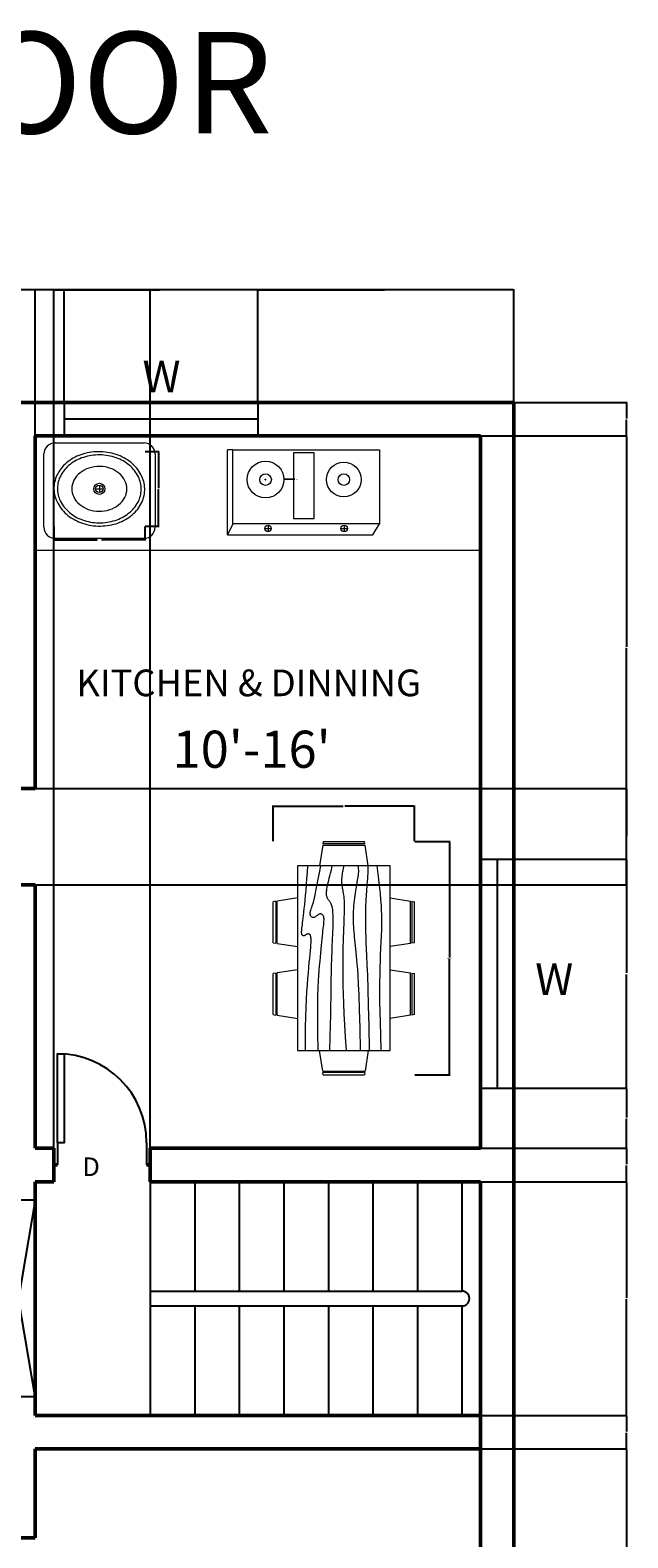
# Model space of a CAD drawing. Units: inches. Extents: x 2164 to 3752, y 2015 to 2629.
# Tile 4 of 8: x 2461 to 2622, y 2223 to 2629. Entities that reach past the tile are written whole.
import ezdxf
from ezdxf.enums import TextEntityAlignment as Align

# ---------------------------------------------------------------- set-up
doc = ezdxf.new("R2010")
doc.units = ezdxf.units.IN
for name, color, linetype, lineweight in [('A-ANNO-DIMS', 2, 'Continuous', 18), ('A-ANNO-TEXT', 7, 'Continuous', 25), ('A-AREA-IDEN', 3, 'Continuous', 25), ('A-DOOR', 3, 'Continuous', 25), ('A-FLOR-FIXT', 8, 'Continuous', 18), ('A-FLOR-STRS', 2, 'Continuous', 25), ('A-FURN', 8, 'Continuous', 18), ('A-GLAZ', 4, 'Continuous', 25), ('A-WALL', 7, 'Continuous', 50)]:
    doc.layers.add(name, color=color, linetype=linetype, lineweight=lineweight)
doc.styles.get("Standard").update_dxf_attribs({"font": 'arial.ttf'})
doc.dimstyles.get("Standard").update_dxf_attribs({"dimtxt": 0.18, "dimasz": 0.18, "dimexe": 0.18, "dimexo": 0.0625, "dimgap": 0.09, "dimtad": 0, "dimtih": 1, "dimtoh": 1, "dimdec": 4, "dimzin": 0, "dimdsep": 46, "dimtxsty": 'Standard', "dimcen": 0.09, "dimadec": 0, "dimazin": 0, "dimtfac": 1, "dimtdec": 4, "dimtofl": 0, "dimtmove": 0, "dimatfit": 3, "dimfxl": 1, "dimtolj": 1, "dimtzin": 0, "dimarcsym": 0})

# ---------------------------------------------------------------- blocks, each defined once
blk = doc.blocks.new('Dining Set - 36 x 72 in.')
for p, q in [((-22.2343, 26.00059), (-23.4847, 17.99762)), ((-22.2304, 26), (-5.7608, 26)), ((-22, 27.5), (-22.1562, 26.50042)), ((-5.8416, 26.5), (-22.1534, 26.5)), ((-22, 27.5), (-6, 27.5)), ((-5.8437, 26.49966), (-6, 27.5)), ((-4.5152, 17.99762), (-5.7655, 25.99926)), ((5.7657, 26.00059), (4.5153, 17.99762)), ((5.7696, 26), (22.2392, 26)), ((6, 27.5), (5.8438, 26.50042)), ((22.1584, 26.5), (5.8466, 26.5)), ((6, 27.5), (22, 27.5)), ((22.1563, 26.49966), (22, 27.5)), ((23.4848, 17.99762), (22.2345, 25.99926)), ((36, 18), (-36, 18)), ((-36, 18), (-36, -18)), ((36, -18), (36, 18)), ((-45.5, 8), (-44.5004, 8.15617)), ((-45.5, 8), (-45.5, -8)), ((-44.5, -8.15843), (-44.5, 8.15338)), ((-44.0006, 8.23428), (-35.9976, 9.48474)), ((-44, 8.23041), (-44, -8.23915)), ((44.0006, 8.23428), (35.9976, 9.48474)), ((44, 8.23041), (44, -8.23915)), ((44.5, -8.15843), (44.5, 8.15338)), ((45.5, 8), (44.5005, 8.15617)), ((45.5, 8), (45.5, -8)), ((-44.4997, -8.15631), (-45.5, -8)), ((-35.9976, -9.48476), (-43.9993, -8.2345)), ((35.9976, -9.48476), (43.9993, -8.2345)), ((44.4997, -8.15631), (45.5, -8)), ((-36, -18), (36, -18)), ((-22.2343, -26.0006), (-23.4847, -17.99762)), ((-4.5152, -17.99762), (-5.7655, -25.99928)), ((5.7657, -26.0006), (4.5153, -17.99762)), ((23.4848, -17.99762), (22.2345, -25.99928)), ((-22.2304, -26), (-5.7608, -26)), ((-22, -27.5), (-22.1562, -26.50044)), ((-5.8416, -26.5), (-22.1534, -26.5)), ((-22, -27.5), (-6, -27.5)), ((-5.8437, -26.49967), (-6, -27.5)), ((5.7696, -26), (22.2392, -26)), ((6, -27.5), (5.8438, -26.50044)), ((22.1584, -26.5), (5.8466, -26.5)), ((6, -27.5), (22, -27.5)), ((22.1563, -26.49967), (22, -27.5))]:
    blk.add_line(p, q)
for points in [[(-36, 15), (-31.1772, 14.97754), (-26.8079, 14.91406), (-22.8538, 14.81543), (-19.276, 14.6875), (-16.0362, 14.53613), (-13.0957, 14.36718), (-10.4159, 14.18652), (-7.9583, 14), (-5.6904, 13.81315), (-3.6035, 13.63021), (-1.6954, 13.45508), (0.0365, 13.29166), (1.5945, 13.14388), (2.9811, 13.01562), (4.1988, 12.9108), (5.25, 12.83333), (6.1393, 12.78613), (6.8802, 12.76823), (7.4883, 12.77767), (7.9792, 12.8125), (8.3685, 12.87077), (8.6719, 12.95052), (8.9049, 13.0498), (9.0833, 13.16666), (9.2205, 13.29899), (9.3216, 13.44401), (9.3895, 13.59879), (9.4271, 13.76041), (9.4373, 13.92594), (9.4232, 14.09245), (9.3875, 14.257), (9.3333, 14.41666), (9.2638, 14.56917), (9.1836, 14.71484), (9.0975, 14.85465), (9.0104, 14.98958), (8.9272, 15.1206), (8.8529, 15.2487), (8.7922, 15.37483), (8.75, 15.5), (8.7305, 15.62467), (8.7344, 15.74739), (8.7617, 15.86621), (8.8125, 15.97916), (8.8867, 16.08431), (8.9844, 16.17968), (9.1055, 16.26334), (9.25, 16.33333), (9.4189, 16.38802), (9.6172, 16.42708), (9.8506, 16.45052), (10.125, 16.45833), (10.4463, 16.45052), (10.8203, 16.42708), (11.2529, 16.38802), (11.75, 16.33333), (12.3184, 16.26318), (12.9694, 16.17838), (13.7151, 16.07991), (14.5677, 15.96875), (15.5395, 15.84586), (16.6426, 15.71224), (17.8893, 15.56884), (19.2917, 15.41666), (20.859, 15.25667), (22.5879, 15.08984), (24.4721, 14.91715), (26.5052, 14.73958), (28.6809, 14.5581), (30.9929, 14.3737), (33.4347, 14.18733), (36, 14)], [(-36, 10), (-28.9766, 10.14274), (-23.1725, 10.20442), (-18.4241, 10.19775), (-14.5677, 10.13541), (-11.4399, 10.03011), (-8.877, 9.89453), (-6.7154, 9.74137), (-4.7917, 9.58333), (-2.9698, 9.43082), (-1.2246, 9.28515), (0.4415, 9.14534), (2.026, 9.01041), (3.5266, 8.87939), (4.9408, 8.7513), (6.266, 8.62516), (7.5, 8.5), (8.6411, 8.37549), (9.6914, 8.2539), (10.6538, 8.13818), (11.5312, 8.03125), (12.3267, 7.93603), (13.043, 7.85547), (13.6831, 7.79248), (14.25, 7.75), (14.7471, 7.7303), (15.1797, 7.73307), (15.5537, 7.75732), (15.875, 7.80208), (16.1494, 7.86637), (16.3828, 7.94922), (16.5811, 8.04964), (16.75, 8.16666), (16.8944, 8.29915), (17.0143, 8.44531), (17.1089, 8.60319), (17.1771, 8.77083), (17.218, 8.94629), (17.2305, 9.1276), (17.2137, 9.31282), (17.1667, 9.5), (17.0895, 9.6875), (16.987, 9.875), (16.8649, 10.0625), (16.7292, 10.25), (16.5856, 10.4375), (16.4401, 10.625), (16.2985, 10.8125), (16.1667, 11), (16.05, 11.18733), (15.9518, 11.3737), (15.8752, 11.5581), (15.8229, 11.73958), (15.798, 11.91715), (15.8034, 12.08984), (15.842, 12.25667), (15.9167, 12.41666), (16.0295, 12.56836), (16.1784, 12.70833), (16.3605, 12.83268), (16.5729, 12.9375), (16.8127, 13.01888), (17.0768, 13.07291), (17.3625, 13.0957), (17.6667, 13.08333), (17.9894, 13.03312), (18.3418, 12.94726), (18.7382, 12.82918), (19.1927, 12.68229), (19.7195, 12.51001), (20.3327, 12.31575), (21.0465, 12.10294), (21.875, 11.875), (22.8357, 11.63354), (23.959, 11.37304), (25.2786, 11.08618), (26.8282, 10.76562), (28.6414, 10.40405), (30.752, 9.99414), (33.1936, 9.52856), (36, 9)], [(-36, 5.5), (-30.7157, 5.3348), (-26.069, 5.20963), (-21.9946, 5.11767), (-18.4271, 5.05208), (-15.3009, 5.00602), (-12.5508, 4.97265), (-10.1112, 4.94515), (-7.9167, 4.91666), (-5.909, 4.88167), (-4.0586, 4.83984), (-2.3429, 4.79215), (-0.7396, 4.73958), (0.7739, 4.6831), (2.22, 4.6237), (3.6213, 4.56233), (5, 4.5), (6.373, 4.43782), (7.7344, 4.3776), (9.0723, 4.32129), (10.375, 4.27083), (11.6309, 4.22819), (12.8281, 4.19531), (13.9551, 4.17415), (15, 4.16666), (15.954, 4.17448), (16.819, 4.19791), (17.6001, 4.23698), (18.3021, 4.29166), (18.9299, 4.36198), (19.4883, 4.44791), (19.9823, 4.54948), (20.4167, 4.66666), (20.7969, 4.79899), (21.1302, 4.94401), (21.4245, 5.09879), (21.6875, 5.26041), (21.9271, 5.42594), (22.1511, 5.59245), (22.3672, 5.757), (22.5834, 5.91666), (22.8065, 6.06868), (23.0404, 6.21093), (23.2879, 6.34147), (23.5521, 6.45833), (23.8358, 6.55957), (24.142, 6.64323), (24.4735, 6.70735), (24.8334, 6.75), (25.2235, 6.76969), (25.642, 6.76692), (26.0858, 6.74267), (26.5521, 6.69791), (27.0379, 6.63362), (27.5404, 6.55078), (28.0565, 6.45036), (28.5834, 6.33333), (29.1242, 6.19987), (29.7071, 6.04687), (30.3661, 5.87044), (31.1354, 5.66666), (32.0493, 5.43164), (33.142, 5.16146), (34.4475, 4.85221), (36, 4.5)], [(-36, -1), (-30.7915, -0.6591), (-26.0195, -0.38216), (-21.6519, -0.16284), (-17.6563, 0.00521), (-14.0005, 0.12833), (-10.6523, 0.21289), (-7.5796, 0.26522), (-4.75, 0.29166), (-2.134, 0.29793), (0.2878, 0.28711), (2.5317, 0.26163), (4.6146, 0.22396), (6.5529, 0.17651), (8.3633, 0.12174), (10.0623, 0.06209), (11.6667, 0), (13.1899, -0.06201), (14.6341, -0.1211), (15.9982, -0.17432), (17.2813, -0.21875), (18.4823, -0.25147), (19.6003, -0.26953), (20.6343, -0.27002), (21.5834, -0.25), (22.4481, -0.20768), (23.2357, -0.14584), (23.9549, -0.06836), (24.6146, 0.02083), (25.2235, 0.11784), (25.7904, 0.21875), (26.3241, 0.31966), (26.8334, 0.41666), (27.3265, 0.50618), (27.8099, 0.58593), (28.2894, 0.65397), (28.7709, 0.70833), (29.2601, 0.74707), (29.763, 0.76823), (30.2855, 0.76985), (30.8334, 0.75), (31.4088, 0.70784), (31.9994, 0.64713), (32.589, 0.57275), (33.1615, 0.48958), (33.7008, 0.4025), (34.1908, 0.3164), (34.6153, 0.23616), (34.9584, 0.16666), (35.2099, 0.11165), (35.3848, 0.07031), (35.504, 0.04069), (35.5886, 0.02083), (35.6594, 0.00879), (35.7377, 0.0026), (35.8442, 0.00032), (36, 0)], [(-36, -6.5), (-27.1843, -6.31267), (-20.084, -6.1263), (-14.469, -5.9419), (-10.1094, -5.76042), (-6.7752, -5.58285), (-4.2363, -5.41016), (-2.2629, -5.24333), (-0.625, -5.08334), (0.8708, -4.93099), (2.2715, -4.78646), (3.5872, -4.64974), (4.8281, -4.52084), (6.0046, -4.39974), (7.127, -4.28646), (8.2053, -4.18099), (9.25, -4.08334), (10.2705, -3.99382), (11.2734, -3.91407), (12.2647, -3.84603), (13.25, -3.79167), (14.2354, -3.75293), (15.2266, -3.73177), (16.2295, -3.73015), (17.25, -3.75), (18.2912, -3.79248), (19.3451, -3.85547), (20.4009, -3.93604), (21.4479, -4.03125), (22.4754, -4.13819), (23.4727, -4.25391), (24.4289, -4.37549), (25.3334, -4.5), (26.1785, -4.62492), (26.9694, -4.74935), (27.7145, -4.87281), (28.4219, -4.99479), (29.1, -5.11483), (29.7572, -5.23242), (30.4016, -5.34709), (31.0417, -5.45834), (31.6837, -5.56437), (32.3262, -5.65821), (32.9658, -5.73153), (33.599, -5.77604), (34.2224, -5.78345), (34.8327, -5.74545), (35.4264, -5.65373), (36, -5.5)], [(-36, -10), (-26.4022, -9.81299), (-18.4675, -9.62891), (-11.9839, -9.45069), (-6.7396, -9.28125), (-2.5226, -9.12354), (0.8789, -8.98047), (3.6769, -8.85498), (6.0833, -8.75), (8.2767, -8.66765), (10.3021, -8.60677), (12.1712, -8.56543), (13.8958, -8.54167), (15.4876, -8.53353), (16.9583, -8.53907), (18.3197, -8.55632), (19.5834, -8.58334), (20.7616, -8.61841), (21.8685, -8.66081), (22.9188, -8.71004), (23.9271, -8.76563), (24.9081, -8.82707), (25.8763, -8.89388), (26.8465, -8.96558), (27.8334, -9.04167), (28.8474, -9.12118), (29.8828, -9.20117), (30.93, -9.27824), (31.9792, -9.34896), (33.0205, -9.40991), (34.0443, -9.45768), (35.0407, -9.48885), (36, -9.5)], [(-36, -14.5), (-30.0881, -14.33513), (-25.0332, -14.21224), (-20.7312, -14.12647), (-17.0781, -14.07292), (-13.97, -14.04671), (-11.3027, -14.04297), (-8.9724, -14.05681), (-6.875, -14.08334), (-4.9224, -14.11833), (-3.0905, -14.16016), (-1.3709, -14.20785), (0.2448, -14.26042), (1.7647, -14.3169), (3.1973, -14.3763), (4.5507, -14.43767), (5.8333, -14.5), (7.0554, -14.5621), (8.235, -14.62175), (9.3922, -14.67652), (10.5469, -14.72396), (11.7192, -14.76164), (12.929, -14.78711), (14.1965, -14.79794), (15.5417, -14.79167), (16.9933, -14.76424), (18.6152, -14.70508), (20.4804, -14.60197), (22.6615, -14.44271), (25.2312, -14.21509), (28.2624, -13.9069), (31.8277, -13.50594), (36, -13)]]:
    blk.add_lwpolyline(points)
blk = doc.blocks.new('Sink - Oval top')
for p, q in [((-1, 0), (1, 0)), ((0, 1), (0, -1))]:
    blk.add_line(p, q)
for points in [[(-12.23, 0.39, 0.117634), (-11.46, -3.36, 0.104469), (-8.88, -6.8, 0.090016), (-5.08, -9.07, 0.08192), (-0.32, -10.02, 0.08192), (4.49, -9.38, 0.090016), (8.42, -7.36, 0.104469), (11.22, -4.09, 0.117634), (12.23, -0.39, 0.117634), (11.46, 3.36, 0.104469), (8.88, 6.8, 0.090016), (5.08, 9.07, 0.08192), (0.32, 10.02, 0.08192), (-4.49, 9.38, 0.090016), (-8.42, 7.36, 0.104469), (-11.22, 4.09, 0.117634)], [(-11.29, 0.16, 0.118622), (-10.52, -3.25, 0.104678), (-8.07, -6.36, 0.089562), (-4.54, -8.37, 0.081185), (-0.13, -9.15, 0.081185), (4.3, -8.49, 0.089562), (7.89, -6.58, 0.104678), (10.42, -3.55, 0.118622), (11.29, -0.16, 0.118622), (10.52, 3.25, 0.104678), (8.07, 6.36, 0.089562), (4.54, 8.37, 0.081185), (0.13, 9.15, 0.081185), (-4.3, 8.49, 0.089562), (-7.89, 6.58, 0.104678), (-10.42, 3.55, 0.118622)], [(-7.42, 0.08, 0.118283), (-6.91, -2.17, 0.104607), (-5.29, -4.21, 0.089718), (-2.97, -5.53, 0.081436), (-0.07, -6.04, 0.081436), (2.84, -5.59, 0.089718), (5.2, -4.33, 0.104607), (6.86, -2.32, 0.118283), (7.42, -0.08, 0.118283), (6.91, 2.17, 0.104607), (5.29, 4.21, 0.089718), (2.97, 5.53, 0.081436), (0.07, 6.04, 0.081436), (-2.84, 5.59, 0.089718), (-5.2, 4.33, 0.104607), (-6.86, 2.32, 0.118283)]]:
    blk.add_lwpolyline(points, format="xyb", close=True)
for radius in [1.5, 1]:
    blk.add_circle((0, 0), radius)
blk = doc.blocks.new('*U2')
for p, q in [((0, 0), (0, -6)), ((24, 0), (24, -6))]:
    blk.add_line(p, q)
blk.add_lwpolyline([(0, 0), (0, 24), (1.75, 24), (1.75, 0)], close=True)
blk.add_arc((0, 0), 24, 0, 90)
blk = doc.blocks.new('STAIR-HANDRAIL')
for p, q in [((84, 63), (84, 33.5)), ((0, 33.5), (84, 33.5)), ((0, 29.5), (84, 29.5)), ((84, 29.5), (84, 0))]:
    blk.add_line(p, q)
blk.add_arc((84, 31.5), 2, 270, 90)
blk = doc.blocks.new('VENT-OPENING')
for p, q in [((9, 53), (0, 53)), ((9, 53), (0, 0)), ((9, 0), (0, 53)), ((9, 0), (0, 0))]:
    blk.add_line(p, q)
blk = doc.blocks.new('*D37')
at = {"layer": 'A-ANNO-DIMS', "color": 0, "lineweight": -2, "transparency": 16777216}
for p, q in [((2564.38, 2410.45), (2573.95, 2410.45)), ((2573.77, 2410.27), (2573.77, 2379.15)), ((2573.77, 2347.66), (2573.77, 2378.78)), ((2564.38, 2347.48), (2573.95, 2347.48))]:
    blk.add_line(p, q, dxfattribs=at)
at = {"layer": 'A-ANNO-DIMS', "color": 0, "transparency": 16777216}
for points in [[(2573.74, 2410.27), (2573.8, 2410.27), (2573.77, 2410.45)], [(2573.74, 2347.66), (2573.8, 2347.66), (2573.77, 2347.48)]]:
    blk.add_solid(points, dxfattribs=at)
at = {"layer": 'Defpoints', "color": 0, "transparency": 16777216}
for p in [(2564.32, 2410.45), (2573.77, 2410.45), (2564.32, 2347.48)]:
    blk.add_point(p, dxfattribs=at)
at = {"layer": 'A-ANNO-DIMS', "color": 0, "transparency": 16777216, "insert": (2573.77, 2378.96), "char_height": 0.18, "attachment_point": 5}
blk.add_mtext('\\A1;DINING SET 63', dxfattribs=at)
blk = doc.blocks.new('*D38')
at = {"layer": 'A-ANNO-DIMS', "color": 0, "lineweight": -2, "transparency": 16777216}
for p, q in [((2526.26, 2410.51), (2526.26, 2420.07)), ((2526.44, 2419.89), (2545.07, 2419.89)), ((2564.14, 2419.89), (2545.51, 2419.89)), ((2564.32, 2410.51), (2564.32, 2420.07))]:
    blk.add_line(p, q, dxfattribs=at)
at = {"layer": 'A-ANNO-DIMS', "color": 0, "transparency": 16777216}
for points in [[(2526.44, 2419.92), (2526.44, 2419.86), (2526.26, 2419.89)], [(2564.14, 2419.92), (2564.14, 2419.86), (2564.32, 2419.89)]]:
    blk.add_solid(points, dxfattribs=at)
at = {"layer": 'Defpoints', "color": 0, "transparency": 16777216}
for p in [(2526.26, 2419.89), (2526.26, 2410.45), (2564.32, 2410.45)]:
    blk.add_point(p, dxfattribs=at)
at = {"layer": 'A-ANNO-DIMS', "color": 0, "transparency": 16777216, "insert": (2545.29, 2419.89), "char_height": 0.18, "attachment_point": 5}
blk.add_mtext('\\A1;38', dxfattribs=at)
blk = doc.blocks.new('*D39')
at = {"layer": 'A-ANNO-DIMS', "color": 0, "lineweight": -2, "transparency": 16777216}
for p, q in [((2467.11, 2495.33), (2467.11, 2491.52)), ((2491.66, 2495.33), (2491.66, 2491.52)), ((2467.29, 2491.7), (2478.83, 2491.7)), ((2491.48, 2491.7), (2479.93, 2491.7))]:
    blk.add_line(p, q, dxfattribs=at)
at = {"layer": 'A-ANNO-DIMS', "color": 0, "transparency": 16777216}
for points in [[(2467.29, 2491.73), (2467.29, 2491.67), (2467.11, 2491.7)], [(2491.48, 2491.73), (2491.48, 2491.67), (2491.66, 2491.7)]]:
    blk.add_solid(points, dxfattribs=at)
at = {"layer": 'Defpoints', "color": 0, "transparency": 16777216}
for p in [(2467.11, 2495.39), (2491.66, 2495.39), (2491.66, 2491.7)]:
    blk.add_point(p, dxfattribs=at)
at = {"layer": 'A-ANNO-DIMS', "color": 0, "transparency": 16777216, "insert": (2479.38, 2491.7), "char_height": 0.18, "attachment_point": 5}
blk.add_mtext('\\A1;SINK 25', dxfattribs=at)
blk = doc.blocks.new('*D40')
at = {"layer": 'A-ANNO-DIMS', "color": 0, "lineweight": -2, "transparency": 16777216}
for p, q in [((2491.72, 2515.52), (2495.52, 2515.52)), ((2495.34, 2515.34), (2495.34, 2505.64)), ((2495.34, 2495.57), (2495.34, 2505.27)), ((2491.72, 2495.39), (2495.52, 2495.39))]:
    blk.add_line(p, q, dxfattribs=at)
at = {"layer": 'A-ANNO-DIMS', "color": 0, "transparency": 16777216}
for points in [[(2495.31, 2515.34), (2495.37, 2515.34), (2495.34, 2515.52)], [(2495.31, 2495.57), (2495.37, 2495.57), (2495.34, 2495.39)]]:
    blk.add_solid(points, dxfattribs=at)
at = {"layer": 'Defpoints', "color": 0, "transparency": 16777216}
for p in [(2491.66, 2515.52), (2495.34, 2515.52), (2491.66, 2495.39)]:
    blk.add_point(p, dxfattribs=at)
at = {"layer": 'A-ANNO-DIMS', "color": 0, "transparency": 16777216, "insert": (2495.34, 2505.46), "char_height": 0.18, "attachment_point": 5}
blk.add_mtext('\\A1;20', dxfattribs=at)
blk = doc.blocks.new('*D51')
at = {"layer": 'A-ANNO-DIMS', "color": 0, "lineweight": -2, "transparency": 16777216}
for p, q in [((2438.92, 2528.78), (2438.92, 2559.25)), ((2439.1, 2559.07), (2453.99, 2559.07)), ((2469.68, 2559.07), (2454.78, 2559.07)), ((2469.86, 2528.78), (2469.86, 2559.25))]:
    blk.add_line(p, q, dxfattribs=at)
at = {"layer": 'A-ANNO-DIMS', "color": 0, "transparency": 16777216}
for points in [[(2439.1, 2559.1), (2439.1, 2559.04), (2438.92, 2559.07)], [(2469.68, 2559.1), (2469.68, 2559.04), (2469.86, 2559.07)]]:
    blk.add_solid(points, dxfattribs=at)
at = {"layer": 'Defpoints', "color": 0, "transparency": 16777216}
for p in [(2469.86, 2559.07), (2438.92, 2528.72), (2469.86, 2528.72)]:
    blk.add_point(p, dxfattribs=at)
at = {"layer": 'A-ANNO-DIMS', "color": 0, "transparency": 16777216, "insert": (2454.39, 2559.07), "char_height": 0.18, "attachment_point": 5}
blk.add_mtext('\\A1;30.94', dxfattribs=at)
blk = doc.blocks.new('*D52')
at = {"layer": 'A-ANNO-DIMS', "color": 0, "lineweight": -2, "transparency": 16777216}
for p, q in [((2469.86, 2528.78), (2469.86, 2559.25)), ((2470.04, 2559.07), (2495.59, 2559.07)), ((2521.89, 2559.07), (2496.34, 2559.07)), ((2522.07, 2528.78), (2522.07, 2559.25))]:
    blk.add_line(p, q, dxfattribs=at)
at = {"layer": 'A-ANNO-DIMS', "color": 0, "transparency": 16777216}
for points in [[(2470.04, 2559.1), (2470.04, 2559.04), (2469.86, 2559.07)], [(2521.89, 2559.1), (2521.89, 2559.04), (2522.07, 2559.07)]]:
    blk.add_solid(points, dxfattribs=at)
at = {"layer": 'Defpoints', "color": 0, "transparency": 16777216}
for p in [(2522.07, 2559.07), (2469.86, 2528.72), (2522.07, 2528.72)]:
    blk.add_point(p, dxfattribs=at)
at = {"layer": 'A-ANNO-DIMS', "color": 0, "transparency": 16777216, "insert": (2495.96, 2559.07), "char_height": 0.18, "attachment_point": 5}
blk.add_mtext('\\A1;52.21', dxfattribs=at)
blk = doc.blocks.new('*D53')
at = {"layer": 'A-ANNO-DIMS', "color": 0, "lineweight": -2, "transparency": 16777216}
for p, q in [((2522.07, 2528.78), (2522.07, 2559.25)), ((2522.25, 2559.07), (2556.2, 2559.07)), ((2590.93, 2559.07), (2556.98, 2559.07)), ((2591.11, 2528.78), (2591.11, 2559.25))]:
    blk.add_line(p, q, dxfattribs=at)
at = {"layer": 'A-ANNO-DIMS', "color": 0, "transparency": 16777216}
for points in [[(2522.25, 2559.1), (2522.25, 2559.04), (2522.07, 2559.07)], [(2590.93, 2559.1), (2590.93, 2559.04), (2591.11, 2559.07)]]:
    blk.add_solid(points, dxfattribs=at)
at = {"layer": 'Defpoints', "color": 0, "transparency": 16777216}
for p in [(2591.11, 2559.07), (2522.07, 2528.72), (2591.11, 2528.72)]:
    blk.add_point(p, dxfattribs=at)
at = {"layer": 'A-ANNO-DIMS', "color": 0, "transparency": 16777216, "insert": (2556.59, 2559.07), "char_height": 0.18, "attachment_point": 5}
blk.add_mtext('\\A1;69.04', dxfattribs=at)
blk = doc.blocks.new('*D54')
at = {"layer": 'A-ANNO-DIMS', "color": 0, "lineweight": -2, "transparency": 16777216}
for p, q in [((2195.11, 2528.78), (2195.11, 2559.25)), ((2195.29, 2559.07), (2392.82, 2559.07)), ((2590.93, 2559.07), (2393.4, 2559.07)), ((2591.11, 2528.78), (2591.11, 2559.25))]:
    blk.add_line(p, q, dxfattribs=at)
at = {"layer": 'A-ANNO-DIMS', "color": 0, "transparency": 16777216}
for points in [[(2195.29, 2559.1), (2195.29, 2559.04), (2195.11, 2559.07)], [(2590.93, 2559.1), (2590.93, 2559.04), (2591.11, 2559.07)]]:
    blk.add_solid(points, dxfattribs=at)
at = {"layer": 'Defpoints', "color": 0, "transparency": 16777216}
for p in [(2591.11, 2559.07), (2195.11, 2528.72), (2591.11, 2528.72)]:
    blk.add_point(p, dxfattribs=at)
at = {"layer": 'A-ANNO-DIMS', "color": 0, "transparency": 16777216, "insert": (2393.11, 2559.07), "char_height": 0.18, "attachment_point": 5}
blk.add_mtext('\\A1;396', dxfattribs=at)
blk = doc.blocks.new('*D58')
at = {"layer": 'A-ANNO-DIMS', "color": 0, "lineweight": -2, "transparency": 16777216}
for p, q in [((2453.11, 2519.78), (2453.11, 2559.25)), ((2453.29, 2559.07), (2457.46, 2559.07)), ((2461.93, 2559.07), (2457.76, 2559.07)), ((2462.11, 2519.78), (2462.11, 2559.25))]:
    blk.add_line(p, q, dxfattribs=at)
at = {"layer": 'A-ANNO-DIMS', "color": 0, "transparency": 16777216}
for points in [[(2453.29, 2559.1), (2453.29, 2559.04), (2453.11, 2559.07)], [(2461.93, 2559.1), (2461.93, 2559.04), (2462.11, 2559.07)]]:
    blk.add_solid(points, dxfattribs=at)
at = {"layer": 'Defpoints', "color": 0, "transparency": 16777216}
for p in [(2462.11, 2559.07), (2453.11, 2519.72), (2462.11, 2519.72)]:
    blk.add_point(p, dxfattribs=at)
at = {"layer": 'A-ANNO-DIMS', "color": 0, "transparency": 16777216, "insert": (2457.61, 2559.07), "char_height": 0.18, "attachment_point": 5}
blk.add_mtext('\\A1;9', dxfattribs=at)
blk = doc.blocks.new('*D79')
at = {"layer": 'A-ANNO-DIMS', "color": 0, "lineweight": -2, "transparency": 16777216}
for p, q in [((2582.17, 2246.72), (2621.64, 2246.72)), ((2621.46, 2246.54), (2621.46, 2206.1)), ((2621.46, 2165.31), (2621.46, 2205.74)), ((2591.17, 2165.13), (2621.64, 2165.13))]:
    blk.add_line(p, q, dxfattribs=at)
at = {"layer": 'A-ANNO-DIMS', "color": 0, "transparency": 16777216}
for points in [[(2621.43, 2246.54), (2621.49, 2246.54), (2621.46, 2246.72)], [(2621.43, 2165.31), (2621.49, 2165.31), (2621.46, 2165.13)]]:
    blk.add_solid(points, dxfattribs=at)
at = {"layer": 'Defpoints', "color": 0, "transparency": 16777216}
for p in [(2582.11, 2246.72), (2621.46, 2246.72), (2591.11, 2165.13)]:
    blk.add_point(p, dxfattribs=at)
at = {"layer": 'A-ANNO-DIMS', "color": 0, "transparency": 16777216, "insert": (2621.46, 2205.92), "char_height": 0.18, "attachment_point": 5}
blk.add_mtext('\\A1;81.59', dxfattribs=at)
blk = doc.blocks.new('*D80')
at = {"layer": 'A-ANNO-DIMS', "color": 0, "lineweight": -2, "transparency": 16777216}
for p, q in [((2582.17, 2255.72), (2621.64, 2255.72)), ((2621.46, 2255.54), (2621.46, 2251.4)), ((2621.46, 2246.9), (2621.46, 2251.04)), ((2582.17, 2246.72), (2621.64, 2246.72))]:
    blk.add_line(p, q, dxfattribs=at)
at = {"layer": 'A-ANNO-DIMS', "color": 0, "transparency": 16777216}
for points in [[(2621.43, 2255.54), (2621.49, 2255.54), (2621.46, 2255.72)], [(2621.43, 2246.9), (2621.49, 2246.9), (2621.46, 2246.72)]]:
    blk.add_solid(points, dxfattribs=at)
at = {"layer": 'Defpoints', "color": 0, "transparency": 16777216}
for p in [(2582.11, 2255.72), (2621.46, 2255.72), (2582.11, 2246.72)]:
    blk.add_point(p, dxfattribs=at)
at = {"layer": 'A-ANNO-DIMS', "color": 0, "transparency": 16777216, "insert": (2621.46, 2251.22), "char_height": 0.18, "attachment_point": 5}
blk.add_mtext('\\A1;9', dxfattribs=at)
blk = doc.blocks.new('*D81')
at = {"layer": 'A-ANNO-DIMS', "color": 0, "lineweight": -2, "transparency": 16777216}
for p, q in [((2582.17, 2318.72), (2621.64, 2318.72)), ((2621.46, 2318.54), (2621.46, 2287.4)), ((2621.46, 2255.9), (2621.46, 2287.04)), ((2582.17, 2255.72), (2621.64, 2255.72))]:
    blk.add_line(p, q, dxfattribs=at)
at = {"layer": 'A-ANNO-DIMS', "color": 0, "transparency": 16777216}
for points in [[(2621.43, 2318.54), (2621.49, 2318.54), (2621.46, 2318.72)], [(2621.43, 2255.9), (2621.49, 2255.9), (2621.46, 2255.72)]]:
    blk.add_solid(points, dxfattribs=at)
at = {"layer": 'Defpoints', "color": 0, "transparency": 16777216}
for p in [(2582.11, 2318.72), (2621.46, 2318.72), (2582.11, 2255.72)]:
    blk.add_point(p, dxfattribs=at)
at = {"layer": 'A-ANNO-DIMS', "color": 0, "transparency": 16777216, "insert": (2621.46, 2287.22), "char_height": 0.18, "attachment_point": 5}
blk.add_mtext('\\A1;63', dxfattribs=at)
blk = doc.blocks.new('*D82')
at = {"layer": 'A-ANNO-DIMS', "color": 0, "lineweight": -2, "transparency": 16777216}
for p, q in [((2582.17, 2327.72), (2621.64, 2327.72)), ((2621.46, 2327.54), (2621.46, 2323.4)), ((2621.46, 2318.9), (2621.46, 2323.04)), ((2582.17, 2318.72), (2621.64, 2318.72))]:
    blk.add_line(p, q, dxfattribs=at)
at = {"layer": 'A-ANNO-DIMS', "color": 0, "transparency": 16777216}
for points in [[(2621.43, 2327.54), (2621.49, 2327.54), (2621.46, 2327.72)], [(2621.43, 2318.9), (2621.49, 2318.9), (2621.46, 2318.72)]]:
    blk.add_solid(points, dxfattribs=at)
at = {"layer": 'Defpoints', "color": 0, "transparency": 16777216}
for p in [(2582.11, 2327.72), (2621.46, 2327.72), (2582.11, 2318.72)]:
    blk.add_point(p, dxfattribs=at)
at = {"layer": 'A-ANNO-DIMS', "color": 0, "transparency": 16777216, "insert": (2621.46, 2323.22), "char_height": 0.18, "attachment_point": 5}
blk.add_mtext('\\A1;9', dxfattribs=at)
blk = doc.blocks.new('*D83')
at = {"layer": 'A-ANNO-DIMS', "color": 0, "lineweight": -2, "transparency": 16777216}
for p, q in [((2591.17, 2343.89), (2621.64, 2343.89)), ((2621.46, 2343.71), (2621.46, 2335.98)), ((2621.46, 2327.9), (2621.46, 2335.62)), ((2582.17, 2327.72), (2621.64, 2327.72))]:
    blk.add_line(p, q, dxfattribs=at)
at = {"layer": 'A-ANNO-DIMS', "color": 0, "transparency": 16777216}
for points in [[(2621.43, 2343.71), (2621.49, 2343.71), (2621.46, 2343.89)], [(2621.43, 2327.9), (2621.49, 2327.9), (2621.46, 2327.72)]]:
    blk.add_solid(points, dxfattribs=at)
at = {"layer": 'Defpoints', "color": 0, "transparency": 16777216}
for p in [(2591.11, 2343.89), (2621.46, 2343.89), (2582.11, 2327.72)]:
    blk.add_point(p, dxfattribs=at)
at = {"layer": 'A-ANNO-DIMS', "color": 0, "transparency": 16777216, "insert": (2621.46, 2335.8), "char_height": 0.18, "attachment_point": 5}
blk.add_mtext('\\A1;16.17', dxfattribs=at)
blk = doc.blocks.new('*D84')
at = {"layer": 'A-ANNO-DIMS', "color": 0, "lineweight": -2, "transparency": 16777216}
for p, q in [((2591.17, 2405.68), (2621.64, 2405.68)), ((2621.46, 2405.5), (2621.46, 2374.97)), ((2621.46, 2344.07), (2621.46, 2374.6)), ((2591.17, 2343.89), (2621.64, 2343.89))]:
    blk.add_line(p, q, dxfattribs=at)
at = {"layer": 'A-ANNO-DIMS', "color": 0, "transparency": 16777216}
for points in [[(2621.43, 2405.5), (2621.49, 2405.5), (2621.46, 2405.68)], [(2621.43, 2344.07), (2621.49, 2344.07), (2621.46, 2343.89)]]:
    blk.add_solid(points, dxfattribs=at)
at = {"layer": 'Defpoints', "color": 0, "transparency": 16777216}
for p in [(2591.11, 2405.68), (2621.46, 2405.68), (2591.11, 2343.89)]:
    blk.add_point(p, dxfattribs=at)
at = {"layer": 'A-ANNO-DIMS', "color": 0, "transparency": 16777216, "insert": (2621.46, 2374.78), "char_height": 0.18, "attachment_point": 5}
blk.add_mtext('\\A1;61.8', dxfattribs=at)
blk = doc.blocks.new('*D85')
at = {"layer": 'A-ANNO-DIMS', "color": 0, "lineweight": -2, "transparency": 16777216}
for p, q in [((2582.17, 2519.72), (2621.64, 2519.72)), ((2621.46, 2519.54), (2621.46, 2462.88)), ((2621.46, 2405.86), (2621.46, 2462.52)), ((2591.17, 2405.68), (2621.64, 2405.68))]:
    blk.add_line(p, q, dxfattribs=at)
at = {"layer": 'A-ANNO-DIMS', "color": 0, "transparency": 16777216}
for points in [[(2621.43, 2519.54), (2621.49, 2519.54), (2621.46, 2519.72)], [(2621.43, 2405.86), (2621.49, 2405.86), (2621.46, 2405.68)]]:
    blk.add_solid(points, dxfattribs=at)
at = {"layer": 'Defpoints', "color": 0, "transparency": 16777216}
for p in [(2582.11, 2519.72), (2621.46, 2519.72), (2591.11, 2405.68)]:
    blk.add_point(p, dxfattribs=at)
at = {"layer": 'A-ANNO-DIMS', "color": 0, "transparency": 16777216, "insert": (2621.46, 2462.7), "char_height": 0.18, "attachment_point": 5}
blk.add_mtext('\\A1;114.04', dxfattribs=at)
blk = doc.blocks.new('*D86')
at = {"layer": 'A-ANNO-DIMS', "color": 0, "lineweight": -2, "transparency": 16777216}
for p, q in [((2591.17, 2528.72), (2621.64, 2528.72)), ((2621.46, 2528.54), (2621.46, 2524.4)), ((2621.46, 2519.9), (2621.46, 2524.04)), ((2582.17, 2519.72), (2621.64, 2519.72))]:
    blk.add_line(p, q, dxfattribs=at)
at = {"layer": 'A-ANNO-DIMS', "color": 0, "transparency": 16777216}
for points in [[(2621.43, 2528.54), (2621.49, 2528.54), (2621.46, 2528.72)], [(2621.43, 2519.9), (2621.49, 2519.9), (2621.46, 2519.72)]]:
    blk.add_solid(points, dxfattribs=at)
at = {"layer": 'Defpoints', "color": 0, "transparency": 16777216}
for p in [(2591.11, 2528.72), (2621.46, 2528.72), (2582.11, 2519.72)]:
    blk.add_point(p, dxfattribs=at)
at = {"layer": 'A-ANNO-DIMS', "color": 0, "transparency": 16777216, "insert": (2621.46, 2524.22), "char_height": 0.18, "attachment_point": 5}
blk.add_mtext('\\A1;9', dxfattribs=at)
blk = doc.blocks.new('*D95')
at = {"layer": 'A-ANNO-DIMS', "color": 0, "lineweight": -2, "transparency": 16777216}
for p, q in [((2467.11, 2327.78), (2467.11, 2559.25)), ((2467.29, 2559.07), (2479.89, 2559.07)), ((2492.93, 2559.07), (2480.33, 2559.07)), ((2493.11, 2327.78), (2493.11, 2559.25))]:
    blk.add_line(p, q, dxfattribs=at)
at = {"layer": 'A-ANNO-DIMS', "color": 0, "transparency": 16777216}
for points in [[(2467.29, 2559.1), (2467.29, 2559.04), (2467.11, 2559.07)], [(2492.93, 2559.1), (2492.93, 2559.04), (2493.11, 2559.07)]]:
    blk.add_solid(points, dxfattribs=at)
at = {"layer": 'Defpoints', "color": 0, "transparency": 16777216}
for p in [(2493.11, 2559.07), (2467.11, 2327.72), (2493.11, 2327.72)]:
    blk.add_point(p, dxfattribs=at)
at = {"layer": 'A-ANNO-DIMS', "color": 0, "transparency": 16777216, "insert": (2480.11, 2559.07), "char_height": 0.18, "attachment_point": 5}
blk.add_mtext('\\A1;26', dxfattribs=at)
blk = doc.blocks.new('*D97')
at = {"layer": 'A-ANNO-DIMS', "color": 0, "lineweight": -2, "transparency": 16777216}
for p, q in [((2462.17, 2424.72), (2621.64, 2424.72)), ((2621.46, 2424.54), (2621.46, 2411.9)), ((2621.46, 2398.9), (2621.46, 2411.54)), ((2462.17, 2398.72), (2621.64, 2398.72))]:
    blk.add_line(p, q, dxfattribs=at)
at = {"layer": 'A-ANNO-DIMS', "color": 0, "transparency": 16777216}
for points in [[(2621.43, 2424.54), (2621.49, 2424.54), (2621.46, 2424.72)], [(2621.43, 2398.9), (2621.49, 2398.9), (2621.46, 2398.72)]]:
    blk.add_solid(points, dxfattribs=at)
at = {"layer": 'Defpoints', "color": 0, "transparency": 16777216}
for p in [(2462.11, 2424.72), (2621.46, 2424.72), (2462.11, 2398.72)]:
    blk.add_point(p, dxfattribs=at)
at = {"layer": 'A-ANNO-DIMS', "color": 0, "transparency": 16777216, "insert": (2621.46, 2411.72), "char_height": 0.18, "attachment_point": 5}
blk.add_mtext('\\A1;26', dxfattribs=at)
blk = doc.blocks.new('*D150')
at = {"layer": 'A-ANNO-DIMS', "color": 0, "lineweight": -2, "transparency": 16777216}
for p, q in [((2524.1, 2507.96), (2524.28, 2507.96)), ((2524.19, 2507.87), (2524.19, 2508.05)), ((2532.11, 2508.03), (2529.32, 2508))]:
    blk.add_line(p, q, dxfattribs=at)
at = {"layer": 'A-ANNO-DIMS', "color": 0, "transparency": 16777216}
blk.add_solid([(2529.32, 2508.03), (2529.32, 2507.97), (2529.14, 2508)], dxfattribs=at)
at = {"layer": 'Defpoints', "color": 0, "transparency": 16777216}
for p in [(2519.23, 2507.91), (2529.14, 2508)]:
    blk.add_point(p, dxfattribs=at)
at = {"layer": 'A-ANNO-DIMS', "color": 0, "transparency": 16777216, "insert": (2532.6, 2508.03), "char_height": 0.18, "attachment_point": 5}
blk.add_mtext('\\A1;∅9.905', dxfattribs=at)

msp = doc.modelspace()

# ---------------------------------------------------------------- linework, layer by layer
at = {"layer": 'A-FLOR-FIXT'}
for p, q in [((2467.4392, 2517.854), (2491.4362, 2517.854)), ((2513.9601, 2493.0794), (2513.9601, 2515.9959)), ((2515.3902, 2515.9959), (2513.9601, 2515.9959)), ((2464.4392, 2495.0883), (2464.4392, 2514.854)), ((2494.4362, 2514.854), (2494.4362, 2495.0883)), ((2531.7072, 2515.1941), (2531.7072, 2497.5087)), ((2537.3015, 2515.1941), (2531.7072, 2515.1941)), ((2537.3015, 2497.5087), (2537.3015, 2515.1941)), ((2515.3902, 2496.0147), (2513.9601, 2493.0794)), ((2524.8551, 2495.6484), (2524.8551, 2493.926)), ((2531.7072, 2497.5087), (2537.3015, 2497.5087)), ((2545.3751, 2495.6484), (2545.3751, 2493.926)), ((2553.1059, 2493.0239), (2554.9364, 2496.0147)), ((2491.4362, 2492.0883), (2467.4392, 2492.0883)), ((2513.9601, 2493.0794), (2553.1059, 2493.0239)), ((2523.9939, 2494.7872), (2525.7163, 2494.7872)), ((2544.5139, 2494.7872), (2546.2363, 2494.7872)), ((2462.1113, 2488.9413), (2582.1113, 2488.9413))]:
    msp.add_line(p, q, dxfattribs=at)
msp.add_lwpolyline([(2515.3902, 2515.9959), (2554.9364, 2515.9959), (2554.9364, 2496.0147), (2515.3902, 2496.0147)], close=True, dxfattribs=at)
for centre, radius in [((2524.187, 2507.955), 4.9523), ((2545.2802, 2507.955), 4.6772), ((2524.187, 2507.955), 1.5591), ((2545.2802, 2507.955), 1.5591), ((2524.8551, 2494.7872), 0.8612), ((2545.3751, 2494.7872), 0.8612)]:
    msp.add_circle(centre, radius, dxfattribs=at)
for centre, start, end in [((2467.4392, 2514.854), 90, 180), ((2491.4362, 2514.854), 0, 90), ((2467.4392, 2495.0883), 180, 270), ((2491.4362, 2495.0883), 270, 0)]:
    msp.add_arc(centre, 3, start, end, dxfattribs=at)
at = {"layer": 'A-FLOR-STRS'}
for p, q in [((2493.1113, 2318.7172), (2493.1113, 2255.7172)), ((2505.1113, 2318.7172), (2505.1113, 2289.2172)), ((2517.1113, 2318.7172), (2517.1113, 2289.2172)), ((2529.1113, 2318.7172), (2529.1113, 2289.2172)), ((2541.1113, 2318.7172), (2541.1113, 2289.2172)), ((2553.1113, 2318.7172), (2553.1113, 2289.2172)), ((2565.1113, 2318.7172), (2565.1113, 2289.2172)), ((2505.1113, 2285.2172), (2505.1113, 2255.7172)), ((2517.1113, 2285.2172), (2517.1113, 2255.7172)), ((2529.1113, 2285.2172), (2529.1113, 2255.7172)), ((2541.1113, 2285.2172), (2541.1113, 2255.7172)), ((2553.1113, 2285.2172), (2553.1113, 2255.7172)), ((2565.1113, 2285.2172), (2565.1113, 2255.7172))]:
    msp.add_line(p, q, dxfattribs=at)
at = {"layer": 'A-GLAZ'}
for p, q in [((2469.8556, 2528.7172), (2469.8556, 2519.7172)), ((2522.0693, 2528.7172), (2522.1113, 2519.7172)), ((2522.0903, 2524.2172), (2469.8556, 2524.2172)), ((2582.1113, 2405.6818), (2591.1113, 2405.6818)), ((2586.6113, 2405.6818), (2586.6113, 2343.8868)), ((2582.1113, 2343.8868), (2591.1113, 2343.8868))]:
    msp.add_line(p, q, dxfattribs=at)
at = {"layer": 'A-WALL'}
for p, q in [((2195.1113, 2528.7172), (2591.1113, 2528.7172)), ((2591.1113, 2528.7172), (2591.1113, 2045.7172)), ((2462.1113, 2519.7172), (2582.1113, 2519.7172)), ((2462.1113, 2519.7172), (2462.1113, 2424.7172)), ((2582.1113, 2519.7172), (2582.1113, 2327.7172)), ((2453.1113, 2424.7172), (2462.1113, 2424.7172)), ((2453.1113, 2398.7172), (2462.1113, 2398.7172)), ((2462.1113, 2398.7172), (2462.1113, 2327.7172)), ((2462.1113, 2332.7172), (2462.1113, 2327.7172)), ((2462.1113, 2327.7172), (2467.1113, 2327.7172)), ((2467.1113, 2327.7172), (2467.1113, 2318.7172)), ((2493.1113, 2323.2172), (2493.1113, 2327.7172)), ((2493.1113, 2327.7172), (2582.1113, 2327.7172)), ((2467.1113, 2323.2172), (2468.1113, 2323.2172)), ((2492.1113, 2323.2172), (2493.1113, 2323.2172)), ((2493.1113, 2323.2172), (2493.1113, 2318.7172)), ((2462.1113, 2318.7172), (2467.1113, 2318.7172)), ((2462.1113, 2318.7172), (2462.1113, 2255.7172)), ((2493.1113, 2318.7172), (2582.1113, 2318.7172)), ((2582.1113, 2318.7172), (2582.1113, 2054.7172)), ((2462.1113, 2255.7172), (2582.1113, 2255.7172)), ((2462.1113, 2246.7172), (2582.1113, 2246.7172)), ((2462.1113, 2246.7172), (2462.1113, 2222.7172)), ((2462.1113, 2222.7172), (2453.1113, 2222.7172))]:
    msp.add_line(p, q, dxfattribs=at)

# ---------------------------------------------------------------- block references
at = {"layer": 'A-DOOR'}
msp.add_blockref('*U2', (2468.1113, 2329.2172), dxfattribs=at)
at = {"layer": 'A-FLOR-FIXT'}
msp.add_blockref('Sink - Oval top', (2479.3817, 2505.4559), dxfattribs=at)
at = {"layer": 'A-FLOR-STRS'}
msp.add_blockref('STAIR-HANDRAIL', (2493.1113, 2255.717), dxfattribs=at)
at = {"layer": 'A-FURN', "xscale": 0.691963255913224, "yscale": 0.691963255913224, "zscale": 0.691963255913224, "rotation": 90}
msp.add_blockref('Dining Set - 36 x 72 in.', (2545.2914, 2378.9621), dxfattribs=at)
at = {"layer": 'A-GLAZ'}
msp.add_blockref('VENT-OPENING', (2453.1113, 2260.717), dxfattribs=at)

# ---------------------------------------------------------------- texts
at = {"layer": 'A-ANNO-TEXT'}
for s, height, p in [('GROUND FLOOR', 27.32215, (2383.759, 2611.4091)), ('W', 8.5558, (2496.1383, 2534.6404)), ('W', 8.5558, (2601.9909, 2372.1703))]:
    msp.add_text(s, height=height, dxfattribs=at).set_placement(p, align=Align.MIDDLE)
msp.add_text('D', height=5, dxfattribs=at).set_placement((2474.82, 2320.251))
at = {"layer": 'A-AREA-IDEN'}
for s, height, p in [('KITCHEN & DINNING ', 7.187671, (2473.1819, 2449.5637)), ("10'-16'", 10, (2499.1341, 2430.2809))]:
    msp.add_text(s, height=height, dxfattribs=at).set_placement(p)

# ---------------------------------------------------------------- dimensions: what is measured, and where the dimension line sits
at = {"layer": 'A-ANNO-DIMS'}
for base, p1, p2, override, picture, middle in [((2591.1113, 2559.0672), (2195.1113, 2528.7172), (2591.1113, 2528.7172), {"dimdec": 0, "dimlfac": 1, "dimrnd": 0, "dimzin": 0, "dimdsep": 46, "dimlunit": 2}, '*D54', (2393.1113, 2559.0672)), ((2469.8556, 2559.0672), (2438.9154, 2528.7172), (2469.8556, 2528.7172), {"dimdec": 2, "dimlfac": 1, "dimrnd": 0, "dimzin": 0, "dimdsep": 46, "dimlunit": 2}, '*D51', (2454.3855, 2559.0672)), ((2462.1113, 2559.0672), (2453.1113, 2519.7172), (2462.1113, 2519.7172), {"dimdec": 0, "dimlfac": 1, "dimrnd": 0, "dimzin": 0, "dimdsep": 46, "dimlunit": 2}, '*D58', (2457.6113, 2559.0672)), ((2493.1113, 2559.0672), (2467.1113, 2327.7172), (2493.1113, 2327.7172), {"dimdec": 0, "dimlfac": 1, "dimrnd": 0, "dimzin": 0, "dimdsep": 46, "dimlunit": 2}, '*D95', (2480.1113, 2559.0672)), ((2522.0693, 2559.0672), (2469.8556, 2528.7172), (2522.0693, 2528.7172), {"dimdec": 2, "dimlfac": 1, "dimrnd": 0, "dimzin": 0, "dimdsep": 46, "dimlunit": 2}, '*D52', (2495.9624, 2559.0672)), ((2591.1113, 2559.0672), (2522.0693, 2528.7172), (2591.1113, 2528.7172), {"dimdec": 2, "dimlfac": 1, "dimrnd": 0, "dimzin": 0, "dimdsep": 46, "dimlunit": 2}, '*D53', (2556.5903, 2559.0672))]:
    dim = msp.add_linear_dim(base=base, p1=p1, p2=p2, dimstyle='Standard', override=override, dxfattribs=at)
    dim.commit()
    dim.dimension.update_dxf_attribs({"geometry": picture, "text_midpoint": middle})
for base, p1, p2, angle, override, picture, middle in [((2621.4613, 2528.7172), (2582.1113, 2519.7172), (2591.1113, 2528.7172), 90, {"dimdec": 0, "dimlfac": 1, "dimrnd": 0, "dimzin": 0, "dimdsep": 46, "dimlunit": 2}, '*D86', (2621.4613, 2524.2172)), ((2621.4613, 2519.7172), (2591.1113, 2405.6818), (2582.1113, 2519.7172), 90, {"dimdec": 2, "dimlfac": 1, "dimrnd": 0, "dimzin": 0, "dimdsep": 46, "dimlunit": 2}, '*D85', (2621.4613, 2462.6995)), ((2495.3398, 2515.5242), (2491.6572, 2495.3876), (2491.6572, 2515.5242), 90, {"dimdec": 0, "dimrnd": 0, "dimzin": 0, "dimlunit": 2}, '*D40', (2495.3398, 2505.4559)), ((2621.4613, 2424.7172), (2462.1113, 2398.7172), (2462.1113, 2424.7172), 90, {"dimdec": 0, "dimlfac": 1, "dimrnd": 0, "dimzin": 0, "dimdsep": 46, "dimlunit": 2}, '*D97', (2621.4613, 2411.7172)), ((2526.2624, 2419.8917), (2564.3204, 2410.4464), (2526.2624, 2410.4464), 180, {"dimdec": 0, "dimrnd": 0, "dimzin": 0, "dimlunit": 2}, '*D38', (2545.2914, 2419.8917)), ((2621.4613, 2405.6818), (2591.1113, 2343.8868), (2591.1113, 2405.6818), 90, {"dimdec": 1, "dimlfac": 1, "dimrnd": 0, "dimzin": 0, "dimdsep": 46, "dimlunit": 2}, '*D84', (2621.4613, 2374.7843)), ((2621.4613, 2343.8868), (2582.1113, 2327.7172), (2591.1113, 2343.8868), 90, {"dimdec": 2, "dimlfac": 1, "dimrnd": 0, "dimzin": 0, "dimdsep": 46, "dimlunit": 2}, '*D83', (2621.4613, 2335.802)), ((2621.4613, 2327.7172), (2582.1113, 2318.7172), (2582.1113, 2327.7172), 90, {"dimdec": 0, "dimlfac": 1, "dimrnd": 0, "dimzin": 0, "dimdsep": 46, "dimlunit": 2}, '*D82', (2621.4613, 2323.2172)), ((2621.4613, 2318.7172), (2582.1113, 2255.7172), (2582.1113, 2318.7172), 90, {"dimdec": 0, "dimlfac": 1, "dimrnd": 0, "dimzin": 0, "dimdsep": 46, "dimlunit": 2}, '*D81', (2621.4613, 2287.2172)), ((2621.4613, 2255.7172), (2582.1113, 2246.7172), (2582.1113, 2255.7172), 90, {"dimdec": 0, "dimlfac": 1, "dimrnd": 0, "dimzin": 0, "dimdsep": 46, "dimlunit": 2}, '*D80', (2621.4613, 2251.2172)), ((2621.4613, 2246.7172), (2591.1113, 2165.1259), (2582.1113, 2246.7172), 90, {"dimdec": 2, "dimlfac": 1, "dimrnd": 0, "dimzin": 0, "dimdsep": 46, "dimlunit": 2}, '*D79', (2621.4613, 2205.9216))]:
    dim = msp.add_linear_dim(base=base, p1=p1, p2=p2, angle=angle, dimstyle='Standard', override=override, dxfattribs=at)
    dim.commit()
    dim.dimension.update_dxf_attribs({"geometry": picture, "text_midpoint": middle})
dim = msp.add_diameter_dim_2p(p1=(2519.2348, 2507.9097), p2=(2529.1391, 2508.0004), dimstyle='Standard', override={"dimdec": 3, "dimlfac": 1, "dimrnd": 0, "dimzin": 0, "dimdsep": 46, "dimlunit": 2}, dxfattribs=at)
dim.commit()
dim.dimension.update_dxf_attribs({"geometry": '*D150', "text_midpoint": (2532.1104, 2508.0276), "dimtype": 163})
dim = msp.add_linear_dim(base=(2491.6572, 2491.705), p1=(2467.1063, 2495.3876), p2=(2491.6572, 2495.3876), text='SINK <>', dimstyle='Standard', override={"dimdec": 0, "dimrnd": 0, "dimzin": 0, "dimlunit": 2}, dxfattribs=at)
dim.commit()
dim.dimension.update_dxf_attribs({"geometry": '*D39', "text_midpoint": (2479.3817, 2491.705)})
dim = msp.add_linear_dim(base=(2573.7657, 2410.4464), p1=(2564.3204, 2347.4778), p2=(2564.3204, 2410.4464), angle=90, text='DINING SET <>', dimstyle='Standard', override={"dimdec": 0, "dimrnd": 0, "dimzin": 0, "dimlunit": 2}, dxfattribs=at)
dim.commit()
dim.dimension.update_dxf_attribs({"geometry": '*D37', "text_midpoint": (2573.7657, 2378.9621)})

doc.saveas('drawing.dxf')
